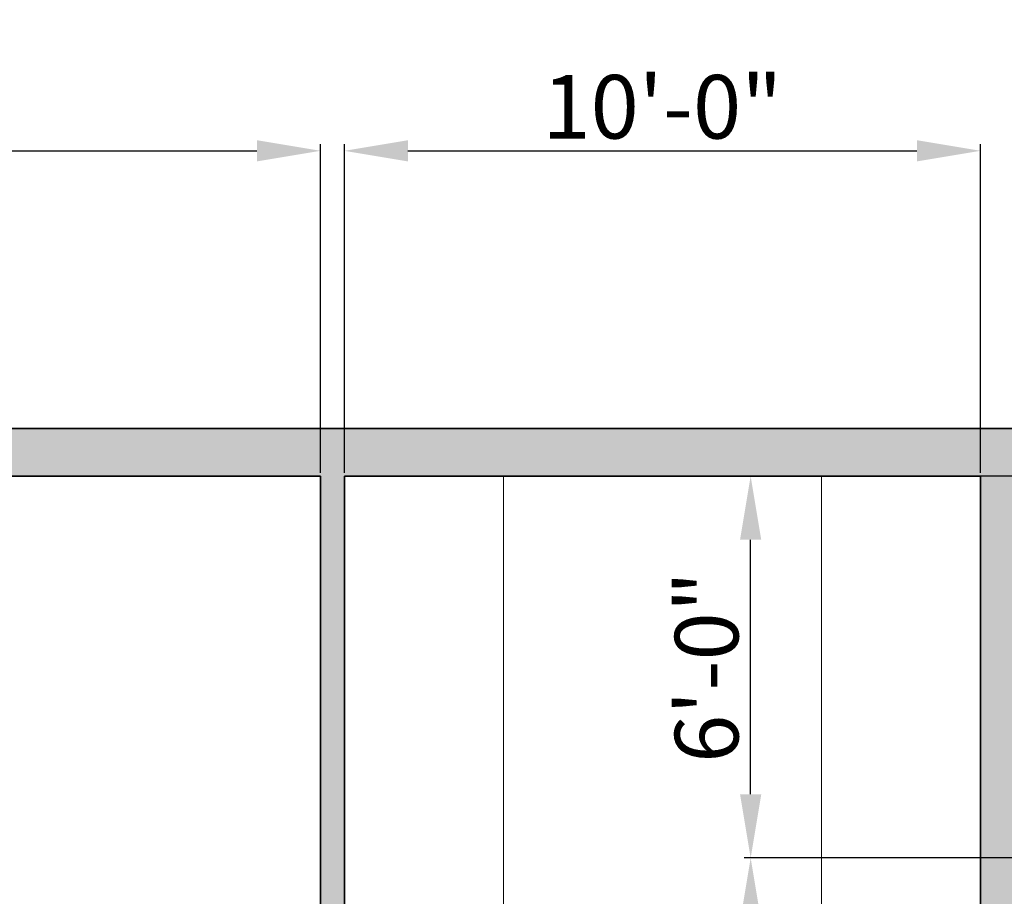
# Model space of a CAD drawing. Units: inches. Extents: x 2083 to 3317, y 1141 to 2115.
# Tile 105 of 256: x 2415 to 2600, y 1933 to 2098. Entities that reach past the tile are written whole.
import ezdxf

# ---------------------------------------------------------------- set-up
doc = ezdxf.new("R2010")
doc.units = ezdxf.units.IN
for name, color, linetype, lineweight in [('A-ANNO-DIMS', 2, 'Continuous', 18), ('A-FLOR-CASE', 8, 'Continuous', 18), ('A-WALL', 7, 'Continuous', 35)]:
    doc.layers.add(name, color=color, linetype=linetype, lineweight=lineweight)
doc.layers.add('A-WALL-PATT', color=251, linetype='Continuous', lineweight=13, true_color=0x636466)
doc.styles.get("Standard").update_dxf_attribs({"font": 'arial.ttf'})
doc.dimstyles.new('ISO-25', dxfattribs={"dimtxt": 12, "dimasz": 12, "dimexe": 1.25, "dimexo": 0.625, "dimtad": 1, "dimlunit": 3, "dimtxsty": 'Standard', "dimcen": 2.5, "dimadec": 0, "dimazin": 0, "dimtfac": 1, "dimtmove": 0, "dimatfit": 3, "dimfxl": 1, "dimarcsym": 0})

# ---------------------------------------------------------------- blocks, each defined once
blk = doc.blocks.new('*D36')
at = {"layer": 'A-ANNO-DIMS', "color": 0, "lineweight": -2, "transparency": 16777216}
for p, q in [((2235.96, 2012.39), (2235.96, 2074.36)), ((2247.96, 2073.11), (2459.46, 2073.11)), ((2471.46, 2012.39), (2471.46, 2074.36))]:
    blk.add_line(p, q, dxfattribs=at)
at = {"layer": 'A-ANNO-DIMS', "color": 0, "transparency": 16777216}
for points in [[(2247.96, 2075.11), (2247.96, 2071.11), (2235.96, 2073.11)], [(2459.46, 2075.11), (2459.46, 2071.11), (2471.46, 2073.11)]]:
    blk.add_solid(points, dxfattribs=at)
at = {"layer": 'Defpoints', "color": 0, "transparency": 16777216}
for p in [(2471.46, 2073.11), (2235.96, 2011.76), (2471.46, 2011.76)]:
    blk.add_point(p, dxfattribs=at)
at = {"layer": 'A-ANNO-DIMS', "color": 0, "transparency": 16777216, "insert": (2353.71, 2079.94), "char_height": 12, "attachment_point": 5}
blk.add_mtext('19\'-7 1/2"', dxfattribs=at)
blk = doc.blocks.new('*D37')
at = {"layer": 'A-ANNO-DIMS', "color": 0, "lineweight": -2, "transparency": 16777216}
for p, q in [((2475.96, 2012.39), (2475.96, 2074.36)), ((2487.96, 2073.11), (2583.96, 2073.11)), ((2595.96, 2012.39), (2595.96, 2074.36))]:
    blk.add_line(p, q, dxfattribs=at)
at = {"layer": 'A-ANNO-DIMS', "color": 0, "transparency": 16777216}
for points in [[(2487.96, 2075.11), (2487.96, 2071.11), (2475.96, 2073.11)], [(2583.96, 2075.11), (2583.96, 2071.11), (2595.96, 2073.11)]]:
    blk.add_solid(points, dxfattribs=at)
at = {"layer": 'Defpoints', "color": 0, "transparency": 16777216}
for p in [(2595.96, 2073.11), (2475.96, 2011.76), (2595.96, 2011.76)]:
    blk.add_point(p, dxfattribs=at)
at = {"layer": 'A-ANNO-DIMS', "color": 0, "transparency": 16777216, "insert": (2535.96, 2079.86), "char_height": 12, "attachment_point": 5}
blk.add_mtext('10\'-0"', dxfattribs=at)
blk = doc.blocks.new('*D50')
at = {"layer": 'A-ANNO-DIMS', "color": 0, "lineweight": -2, "transparency": 16777216}
for p, q in [((2604.33, 1939.76), (2551.36, 1939.76)), ((2552.61, 1807.76), (2552.61, 1927.76)), ((2604.33, 1795.76), (2551.36, 1795.76))]:
    blk.add_line(p, q, dxfattribs=at)
at = {"layer": 'A-ANNO-DIMS', "color": 0, "transparency": 16777216}
for points in [[(2550.61, 1927.76), (2554.61, 1927.76), (2552.61, 1939.76)], [(2550.61, 1807.76), (2554.61, 1807.76), (2552.61, 1795.76)]]:
    blk.add_solid(points, dxfattribs=at)
at = {"layer": 'Defpoints', "color": 0, "transparency": 16777216}
for p in [(2552.61, 1939.76), (2604.96, 1939.76), (2604.96, 1795.76)]:
    blk.add_point(p, dxfattribs=at)
at = {"layer": 'A-ANNO-DIMS', "color": 0, "transparency": 16777216, "insert": (2545.86, 1867.76), "char_height": 12, "attachment_point": 5, "rotation": 90}
blk.add_mtext('12\'-0"', dxfattribs=at)
blk = doc.blocks.new('*D51')
at = {"layer": 'A-ANNO-DIMS', "color": 0, "lineweight": -2, "transparency": 16777216}
for p, q in [((2604.33, 2011.76), (2551.36, 2011.76)), ((2552.61, 1951.76), (2552.61, 1999.76)), ((2604.33, 1939.76), (2551.36, 1939.76))]:
    blk.add_line(p, q, dxfattribs=at)
at = {"layer": 'A-ANNO-DIMS', "color": 0, "transparency": 16777216}
for points in [[(2550.61, 1999.76), (2554.61, 1999.76), (2552.61, 2011.76)], [(2550.61, 1951.76), (2554.61, 1951.76), (2552.61, 1939.76)]]:
    blk.add_solid(points, dxfattribs=at)
at = {"layer": 'Defpoints', "color": 0, "transparency": 16777216}
for p in [(2552.61, 2011.76), (2604.96, 2011.76), (2604.96, 1939.76)]:
    blk.add_point(p, dxfattribs=at)
at = {"layer": 'A-ANNO-DIMS', "color": 0, "transparency": 16777216, "insert": (2545.86, 1975.76), "char_height": 12, "attachment_point": 5, "rotation": 90}
blk.add_mtext('6\'-0"', dxfattribs=at)

msp = doc.modelspace()

# ---------------------------------------------------------------- hatches: boundary and pattern name
at = {"layer": 'A-WALL-PATT'}
h = msp.add_hatch(color=256, dxfattribs=at)
h.dxf.hatch_style = 1
h.paths.add_polyline_path([(3126.96, 2020.761), (2748.96, 2020.761), (2604.96, 2020.761), (2226.96, 2020.761), (2226.96, 1702.761), (2466.96, 1702.761), (2466.96, 1582.761), (2418.96, 1582.761), (2418.96, 1477.761), (2226.96, 1477.761), (2226.96, 1263.261), (2544.96, 1263.261), (2544.96, 1411.761), (2604.96, 1411.761), (2685.96, 1411.761), (2685.96, 1420.761), (2604.96, 1420.761), (2604.96, 1573.761), (2604.96, 1702.761), (2604.96, 2011.761), (2748.96, 2011.761), (2748.96, 1702.761), (2862.96, 1702.761), (2862.96, 1621.761), (2871.96, 1621.761), (2871.96, 1702.761), (2883.96, 1702.761), (2883.96, 1706.939, -0.0264593), (2883.96, 1711.761), (2757.96, 1711.761), (2757.96, 1807.761), (2787.96, 1807.761), (2787.96, 1812.261), (2757.96, 1812.261), (2757.96, 2011.761), (2877.96, 2011.761), (2877.96, 1812.261), (2847.96, 1812.261), (2847.96, 1807.761), (2889.836, 1807.761), (2889.836, 1812.261), (2882.46, 1812.261), (2882.46, 2011.761), (3117.96, 2011.761), (3117.96, 1812.261), (2937.836, 1812.261), (2937.836, 1807.761), (2995.71, 1807.761), (2995.71, 1796.118), (3000.21, 1796.118), (3000.21, 1807.761), (3117.96, 1807.761), (3117.96, 1711.761), (3000.21, 1711.761), (3000.21, 1760.118), (2998.573, 1760.118, -0.020711), (2995.71, 1760.118), (2995.71, 1711.761), (2931.96, 1711.761), (2931.96, 1702.761), (3126.96, 1702.761)])
h.paths.add_polyline_path([(2471.46, 2011.761), (2471.46, 1810.011), (2462.717, 1810.011), (2462.717, 1805.511), (2505.96, 1805.511), (2505.96, 1810.011), (2475.96, 1810.011), (2475.96, 2011.761), (2595.96, 2011.761), (2595.96, 1810.011), (2565.96, 1810.011), (2565.96, 1805.511), (2595.96, 1805.511), (2595.96, 1711.761), (2235.96, 1711.761), (2235.96, 1805.511), (2353.71, 1805.511), (2353.71, 1796.054), (2358.21, 1796.054), (2358.21, 1805.511), (2414.717, 1805.511), (2414.717, 1810.011), (2235.96, 1810.011), (2235.96, 2011.761)], flags=16)
h.paths.add_polyline_path([(2270.205, 1994.61), (2270.205, 1970.61), (2246.205, 1970.61), (2246.205, 1994.61)], flags=0)
edge = h.paths.add_edge_path(flags=0)
edge.add_ellipse((2332.027, 1899.798), major_axis=(-3.043, 3.043), ratio=0.1682525, start_angle=-161.33217, end_angle=-156.30711, ccw=False)
edge.add_ellipse((2333.082, 1898.744), major_axis=(-1.055, 1.055), ratio=0.4535321, start_angle=-123.37102, end_angle=-94.15911)
edge = h.paths.add_edge_path(flags=0)
edge.add_ellipse((2332.027, 1968.876), major_axis=(3.043, 3.043), ratio=0.1682525, start_angle=18.66783, end_angle=23.69289)
edge.add_spline(control_points=[(2332.926, 1970.691), (2332.227, 1970.336), (2330.894, 1969.659), (2328.413, 1970.932), (2327.204, 1967.749), (2324.71, 1969.956), (2322.533, 1967.012), (2320.013, 1971.296), (2317.68, 1968.158), (2316.041, 1967.102), (2315.427, 1966.81)], knot_values=[0, 0, 0, 0, 2.2670587, 4.3245589, 6.6855835, 8.8786411, 11.121502, 14.300359, 17.7552837, 19.732645, 19.732645, 19.732645, 19.732645], degree=3, periodic=0)
edge.add_ellipse((2332.027, 1968.876), major_axis=(3.043, 3.043), ratio=0.1682525, start_angle=18.66783, end_angle=23.69289, ccw=False)
edge.add_ellipse((2333.082, 1969.931), major_axis=(1.055, 1.055), ratio=0.4535321, start_angle=56.62898, end_angle=85.84089, ccw=False)
edge = h.paths.add_edge_path(flags=0)
edge.add_spline(control_points=[(2296.428, 1967.988), (2293.628, 1965.336), (2287.704, 1959.727), (2299.744, 1949.996), (2294.533, 1935.669), (2290.573, 1920.604), (2293.394, 1909.974), (2296.185, 1904.967)], knot_values=[0.0991853, 0.0991853, 0.0991853, 0.0991853, 0.3453009, 0.6198217, 0.9826526, 1.3860932, 1.8105546, 1.8105546, 1.8105546, 1.8105546], degree=3, periodic=0)
edge.add_spline(control_points=[(2296.185, 1904.967), (2297.384, 1902.619), (2298.001, 1901.949), (2298.553, 1901.468)], knot_values=[0.0062457, 0.0062457, 0.0062457, 0.0062457, 0.0554759, 0.0554759, 0.0554759, 0.0554759], degree=3, periodic=0)
edge.add_spline(control_points=[(2298.553, 1901.468), (2297.259, 1900.923), (2295.225, 1900.232), (2293.06, 1900.614), (2292.101, 1900.788), (2292.09, 1900.791)], knot_values=[0.3128349, 0.3128349, 0.3128349, 0.3128349, 0.4017797, 0.4749867, 0.4759027, 0.4759027, 0.4759027, 0.4759027], degree=3, periodic=0)
edge.add_arc((2292.794, 1904.664), 3.937, 215.4209, 259.69818, ccw=False)
edge.add_spline(control_points=[(2289.585, 1902.382), (2289.477, 1902.535), (2289.368, 1902.688), (2289.261, 1902.841)], knot_values=[0.1028719, 0.1028719, 0.1028719, 0.1028719, 0.1168958, 0.1168958, 0.1168958, 0.1168958], degree=3, periodic=0)
edge.add_spline(control_points=[(2289.261, 1902.841), (2288.687, 1902.55), (2287.64, 1902.02), (2285.881, 1901.874), (2283.853, 1901.504), (2281.72, 1899.711), (2278.467, 1899.493), (2276.157, 1901.883), (2272.259, 1899.804), (2267.778, 1901.843), (2262.244, 1900.184), (2257.415, 1901.782), (2254.318, 1900.726), (2253.178, 1900.337)], knot_values=[0, 0, 0, 0, 1.9079767, 3.4771759, 5.261074, 7.9728515, 11.6802485, 13.7179214, 16.9395917, 22.789562, 27.5025027, 33.5952153, 37.1456181, 37.1456181, 37.1456181, 37.1456181], degree=3, periodic=0)
edge.add_line((2253.178, 1900.337), (2250.244, 1902.841))
edge.add_line((2250.244, 1902.841), (2250.244, 1965.833))
edge.add_line((2250.244, 1965.833), (2253.178, 1968.337))
edge.add_spline(control_points=[(2253.178, 1968.337), (2254.318, 1967.948), (2257.415, 1966.892), (2262.244, 1968.49), (2267.778, 1966.831), (2271.527, 1968.537), (2273.876, 1967.828), (2274.207, 1967.728)], knot_values=[0, 0, 0, 0, 0.0901802, 0.2449351, 0.3646438, 0.5132331, 0.5378548, 0.5378548, 0.5378548, 0.5378548], degree=3, periodic=0)
edge.add_arc((2274.353, 1963.793), 3.937, 72.05113, 92.12795, ccw=False)
edge.add_arc((2281.297, 1985.23), 18.596, 252.05113, 288.56572)
edge.add_arc((2292.317, 1956.029), 12.646, 71.02679, 113.77822, ccw=False)
edge = h.paths.add_edge_path(flags=0)
edge.add_spline(control_points=[(2274.899, 1951.856), (2275.066, 1951.617), (2275.233, 1951.377), (2275.398, 1951.136)], knot_values=[1.4099157, 1.4099157, 1.4099157, 1.4099157, 1.4315903, 1.4315903, 1.4315903, 1.4315903], degree=3, periodic=0)
edge.add_spline(control_points=[(2275.398, 1951.136), (2275.792, 1950.562), (2276.179, 1949.984), (2276.546, 1949.397)], knot_values=[1.3582378, 1.3582378, 1.3582378, 1.3582378, 1.4099157, 1.4099157, 1.4099157, 1.4099157], degree=3, periodic=0)
edge.add_line((2276.546, 1949.397), (2277.437, 1947.862))
edge.add_spline(control_points=[(2277.437, 1947.862), (2276.304, 1945.673), (2274.64, 1942.427), (2274.632, 1938.094), (2272.799, 1930.852), (2274.356, 1943.897), (2275.948, 1947.923), (2276.546, 1949.397)], knot_values=[0.0056315, 0.0056315, 0.0056315, 0.0056315, 0.1860139, 0.2660015, 0.3570872, 0.5963902, 0.7397317, 0.7397317, 0.7397317, 0.7397317], degree=3, periodic=0)
edge.add_spline(control_points=[(2276.546, 1949.397), (2276.179, 1949.984), (2275.792, 1950.562), (2275.398, 1951.136)], knot_values=[1.3582378, 1.3582378, 1.3582378, 1.3582378, 1.4099157, 1.4099157, 1.4099157, 1.4099157], degree=3, periodic=0)
edge.add_spline(control_points=[(2275.398, 1951.136), (2274.943, 1950.08), (2274.208, 1948.025), (2273.935, 1944.851), (2272.469, 1937.627), (2273.466, 1945.696), (2274.701, 1951.059), (2274.899, 1951.856)], knot_values=[0.1043639, 0.1043639, 0.1043639, 0.1043639, 0.1896363, 0.2696239, 0.3607096, 0.6000126, 0.6446217, 0.6446217, 0.6446217, 0.6446217], degree=3, periodic=0)
h.paths.add_polyline_path([(2269.168, 1963.128, -0.3575267), (2268.171, 1960.976, -0.0925607), (2268.171, 1939.436, -0.3575267), (2269.168, 1937.285, -0.3575267), (2267.016, 1938.282, -0.1647847), (2254.686, 1938.282, -0.3575267), (2252.534, 1937.285, -0.3575267), (2253.531, 1939.436, -0.0925607), (2253.531, 1960.976, -0.3575267), (2252.534, 1963.128, -0.3575267), (2254.686, 1962.131, -0.1647847), (2267.016, 1962.131, -0.3575267)], flags=0)
h.paths.add_polyline_path([(2248.874, 1967.802), (2248.874, 1957.028), (2249.458, 1957.028), (2249.458, 1911.647), (2248.874, 1911.647), (2248.874, 1900.873), (2246.512, 1900.873, 0.1973271), (2244.15, 1902.457), (2244.15, 1966.218, 0.1973271), (2246.512, 1967.802)], flags=0)
h.paths.add_polyline_path([(2269.168, 1931.389, -0.3575267), (2268.171, 1929.238, -0.0925607), (2268.171, 1907.698, -0.3575267), (2269.168, 1905.547, -0.3575267), (2267.016, 1906.544, -0.1647847), (2254.686, 1906.544, -0.3575267), (2252.534, 1905.547, -0.3575267), (2253.531, 1907.698, -0.0925607), (2253.531, 1929.238, -0.3575267), (2252.534, 1931.389, -0.3575267), (2254.686, 1930.392, -0.1647847), (2267.016, 1930.392, -0.3575267)], flags=0)
edge = h.paths.add_edge_path(flags=0)
edge.add_spline(control_points=[(2276.197, 1906.724), (2276.168, 1909.029), (2276.114, 1913.372), (2270.598, 1924.925), (2273.905, 1919.013), (2275.922, 1916.262), (2275.475, 1912.402), (2277.258, 1910.381), (2276.696, 1908.225), (2276.646, 1906.813), (2276.618, 1906.008)], knot_values=[0, 0, 0, 0, 8.6102597, 16.2212739, 18.8430575, 23.8048978, 27.4408283, 29.3561016, 31.2034776, 33.6506866, 33.6506866, 33.6506866, 33.6506866], degree=3, periodic=0)
edge.add_spline(control_points=[(2276.618, 1906.008), (2276.623, 1905.624), (2276.498, 1904.629), (2275.442, 1903.855), (2274.937, 1903.08), (2274.859, 1902.841)], knot_values=[0.1564884, 0.1564884, 0.1564884, 0.1564884, 0.1843975, 0.2313765, 0.2505985, 0.2505985, 0.2505985, 0.2505985], degree=3, periodic=0)
edge.add_line((2274.859, 1902.841), (2276.506, 1902.841))
edge.add_spline(control_points=[(2276.506, 1902.841), (2276.788, 1903.085), (2277.665, 1904.125), (2278.25, 1904.341), (2277.654, 1908.527), (2278.156, 1906.228), (2278.1, 1905.286), (2278.847, 1904.069), (2277.857, 1903.415), (2277.874, 1902.991), (2277.904, 1902.841)], knot_values=[0.0595743, 0.0595743, 0.0595743, 0.0595743, 0.0807529, 0.1037415, 0.1697201, 0.1760361, 0.2071372, 0.2404744, 0.2623409, 0.2736605, 0.2736605, 0.2736605, 0.2736605], degree=3, periodic=0)
edge.add_line((2277.904, 1902.841), (2280.03, 1902.841))
edge.add_spline(control_points=[(2280.03, 1902.841), (2279.888, 1903.088), (2279.499, 1903.982), (2280.152, 1905.939), (2278.104, 1909.658), (2279.762, 1907.185), (2280.328, 1904.875), (2280.485, 1903.49), (2281.463, 1903.249), (2281.758, 1902.936), (2281.834, 1902.841)], knot_values=[0.013856, 0.013856, 0.013856, 0.013856, 0.0348738, 0.0888667, 0.1078792, 0.1267378, 0.158714, 0.1937575, 0.2174868, 0.2267221, 0.2267221, 0.2267221, 0.2267221], degree=3, periodic=0)
edge.add_spline(control_points=[(2281.834, 1902.841), (2281.788, 1902.827), (2281.647, 1902.783), (2281.396, 1902.859), (2281.088, 1902.985), (2280.721, 1903.061), (2280.333, 1903.026), (2280.125, 1902.899), (2280.03, 1902.841)], knot_values=[0, 0, 0, 0, 0.1441304, 0.435517, 0.7492759, 1.1530457, 1.5483707, 1.878348, 1.878348, 1.878348, 1.878348], degree=3, periodic=0)
edge.add_line((2280.03, 1902.841), (2277.904, 1902.841))
edge.add_spline(control_points=[(2277.904, 1902.841), (2277.893, 1902.796), (2277.865, 1902.68), (2277.607, 1902.687), (2277.274, 1902.801), (2276.838, 1902.62), (2276.584, 1902.789), (2276.506, 1902.841)], knot_values=[0, 0, 0, 0, 0.1271885, 0.3261988, 0.6280094, 1.2435704, 1.5153306, 1.5153306, 1.5153306, 1.5153306], degree=3, periodic=0)
edge.add_line((2276.506, 1902.841), (2274.859, 1902.841))
edge.add_spline(control_points=[(2274.859, 1902.841), (2274.814, 1902.899), (2274.725, 1903.013), (2274.493, 1903.119), (2274.244, 1902.961), (2273.937, 1903.185), (2273.614, 1902.983), (2273.408, 1902.883), (2273.322, 1902.841)], knot_values=[0, 0, 0, 0, 0.2184302, 0.4369566, 0.6879766, 0.9903786, 1.3983955, 1.6918498, 1.6918498, 1.6918498, 1.6918498], degree=3, periodic=0)
edge.add_spline(control_points=[(2273.322, 1902.841), (2273.617, 1903.446), (2274.274, 1904.538), (2276.027, 1904.574), (2276.207, 1906.584), (2276.197, 1906.724)], knot_values=[0.0122268, 0.0122268, 0.0122268, 0.0122268, 0.0594721, 0.1062177, 0.134458, 0.134458, 0.134458, 0.134458], degree=3, periodic=0)
h.paths.add_polyline_path([(2270.776, 1897.79), (2270.776, 1873.79), (2246.776, 1873.79), (2246.776, 1897.79)], flags=0)
h.paths.add_polyline_path([(2353.71, 1760.005), (2353.71, 1760.054), (2358.21, 1760.054, -0.033729)], flags=0)
h.paths.add_polyline_path([(2321.819, 1737.529), (2341.995, 1737.529, -0.4142136), (2343.203, 1736.321), (2343.203, 1721.021, -0.4142136), (2341.995, 1719.813), (2321.819, 1719.813, -0.4142136), (2320.611, 1721.021), (2320.611, 1736.321, -0.4142136)], flags=0)
h.paths.add_polyline_path([(2324.235, 1736.321), (2339.579, 1736.321, -0.4142136), (2341.995, 1733.905), (2341.995, 1725.45, -0.4142136), (2339.579, 1723.034), (2333.681, 1723.034), (2333.845, 1722.045, -0.8706461), (2335.425, 1721.826, -0.767327), (2333.923, 1721.423), (2331.291, 1721.423, -0.767327), (2329.788, 1721.826, -0.8706461), (2331.368, 1722.045), (2331.533, 1723.034), (2324.235, 1723.034, -0.4142136), (2321.819, 1725.45), (2321.819, 1733.905, -0.4142136)], flags=0)
h.paths.add_polyline_path([(2570.484, 1928.615), (2589.684, 1928.615), (2590.169, 1928.615), (2590.169, 1904.993), (2570.484, 1904.993)], flags=0)
h.paths.add_polyline_path([(2574.447, 1927.264, -1), (2572.829, 1927.264, -1)], flags=0)
h.paths.add_polyline_path([(2573.09, 1926.941), (2573.925, 1927.776), (2574.148, 1927.553), (2573.313, 1926.718)], flags=0)
h.paths.add_polyline_path([(2578.779, 1919.73, -1), (2571.592, 1919.73, -1)], flags=0)
h.paths.add_polyline_path([(2578.385, 1919.73, -1), (2571.985, 1919.73, -1)], flags=0)
h.paths.add_polyline_path([(2331.596, 1729.476, -1), (2333.618, 1729.476, -1)], flags=0)
h.paths.add_polyline_path([(2578.034, 1927.264, -1), (2576.416, 1927.264, -1)], flags=0)
h.paths.add_polyline_path([(2576.689, 1927.531), (2576.912, 1927.754), (2577.747, 1926.919), (2577.524, 1926.696)], flags=0)
h.paths.add_polyline_path([(2578.139, 1909.86, -1), (2572.232, 1909.86, -1)], flags=0)
h.paths.add_polyline_path([(2577.745, 1909.86, -1), (2572.625, 1909.86, -1)], flags=0)
h.paths.add_polyline_path([(2583.798, 1927.264, -1), (2582.179, 1927.264, -1)], flags=0)
h.paths.add_polyline_path([(2582.719, 1927.754), (2583.554, 1926.919), (2583.331, 1926.696), (2582.496, 1927.531)], flags=0)
h.paths.add_polyline_path([(2582.496, 1927.531), (2582.719, 1927.754), (2583.554, 1926.919), (2583.331, 1926.696)], flags=0)
h.paths.add_polyline_path([(2587.739, 1920.53, -1), (2581.832, 1920.53, -1)], flags=0)
h.paths.add_polyline_path([(2587.345, 1920.53, -1), (2582.225, 1920.53, -1)], flags=0)
h.paths.add_polyline_path([(2587.385, 1927.264, -1), (2585.766, 1927.264, -1)], flags=0)
h.paths.add_polyline_path([(2586.082, 1926.98), (2586.917, 1927.815), (2587.14, 1927.593), (2586.305, 1926.758)], flags=0)
h.paths.add_polyline_path([(2588.379, 1910.66, -1), (2581.192, 1910.66, -1)], flags=0)
h.paths.add_polyline_path([(2587.985, 1910.66, -1), (2581.585, 1910.66, -1)], flags=0)
h.paths.add_polyline_path([(2417.168, 1729.478), (2437.344, 1729.478, -0.4142136), (2438.552, 1728.27), (2438.552, 1712.969, -0.4142136), (2437.344, 1711.761), (2417.168, 1711.761, -0.4142136), (2415.96, 1712.969), (2415.96, 1728.27, -0.4142136)], flags=0)
h.paths.add_polyline_path([(2419.584, 1728.27), (2434.928, 1728.27, -0.4142136), (2437.344, 1725.854), (2437.344, 1717.398, -0.4142136), (2434.928, 1714.983), (2429.029, 1714.983), (2429.194, 1713.994, -0.8706461), (2430.774, 1713.775, -0.767327), (2429.271, 1713.372), (2426.64, 1713.372, -0.767327), (2425.137, 1713.775, -0.8706461), (2426.717, 1713.994), (2426.882, 1714.983), (2419.584, 1714.983, -0.4142136), (2417.168, 1717.398), (2417.168, 1725.854, -0.4142136)], flags=0)
h.paths.add_polyline_path([(2419.584, 1728.27), (2434.928, 1728.27, -0.4142136), (2437.344, 1725.854), (2437.344, 1717.398, -0.4142136), (2434.928, 1714.983), (2429.029, 1714.983), (2428.358, 1719.009), (2427.553, 1719.009), (2426.882, 1714.983), (2419.584, 1714.983, -0.4142136), (2417.168, 1717.398), (2417.168, 1725.854, -0.4142136)], flags=0)
h.paths.add_polyline_path([(2426.944, 1721.425, -1), (2428.967, 1721.425, -1)], flags=0)
h.paths.add_polyline_path([(2475.96, 1702.761), (2595.96, 1702.761), (2595.96, 1582.761), (2475.96, 1582.761)], flags=16)
h.paths.add_polyline_path([(2427.96, 1573.761), (2595.96, 1573.761), (2595.96, 1468.761), (2595.96, 1420.761), (2384.46, 1420.761), (2384.46, 1468.761), (2427.96, 1468.761)], flags=16)
h.paths.add_polyline_path([(2379.96, 1468.761), (2379.96, 1420.761), (2235.96, 1420.761), (2235.96, 1468.761)], flags=16)
h.paths.add_polyline_path([(2317.816, 1466.696), (2337.992, 1466.696, -0.4142136), (2339.2, 1465.488), (2339.2, 1450.187, -0.4142136), (2337.992, 1448.979), (2317.816, 1448.979, -0.4142136), (2316.608, 1450.187), (2316.608, 1465.488, -0.4142136)], flags=0)
h.paths.add_polyline_path([(2320.232, 1465.488), (2335.576, 1465.488, -0.4142136), (2337.992, 1463.072), (2337.992, 1454.616, -0.4142136), (2335.576, 1452.2), (2329.677, 1452.2), (2329.842, 1451.212, -0.8706461), (2331.422, 1450.992, -0.767327), (2329.92, 1450.59), (2327.288, 1450.59, -0.767327), (2325.785, 1450.992, -0.8706461), (2327.365, 1451.212), (2327.53, 1452.2), (2320.232, 1452.2, -0.4142136), (2317.816, 1454.616), (2317.816, 1463.072, -0.4142136)], flags=0)
h.paths.add_polyline_path([(2320.232, 1465.488), (2335.576, 1465.488, -0.4142136), (2337.992, 1463.072), (2337.992, 1454.616, -0.4142136), (2335.576, 1452.2), (2329.677, 1452.2), (2329.006, 1456.227), (2328.201, 1456.227), (2327.53, 1452.2), (2320.232, 1452.2, -0.4142136), (2317.816, 1454.616), (2317.816, 1463.072, -0.4142136)], flags=0)
h.paths.add_polyline_path([(2327.593, 1458.643, -1), (2329.615, 1458.643, -1)], flags=0)
h.paths.add_polyline_path([(2244.412, 1433.34), (2241.921, 1433.34, -0.4142136), (2240.018, 1435.244), (2240.018, 1440.953, -0.4142105), (2241.921, 1442.856), (2244.412, 1442.856, -1.9764724)], flags=0)
h.paths.add_polyline_path([(2245.357, 1434.398, -0.4142136), (2245.357, 1441.799, -2.1440985)], flags=0)
h.paths.add_polyline_path([(2535.96, 1416.261), (2535.96, 1272.261), (2235.96, 1272.261), (2235.96, 1416.261)], flags=16)
h.paths.add_polyline_path([(2260.12, 1384.293), (2260.12, 1362.039), (2237.865, 1362.039), (2237.865, 1384.293)], flags=0)
edge = h.paths.add_edge_path(flags=0)
edge.add_line((2318.252, 1362.093), (2318.146, 1362.001))
edge.add_ellipse((2317.445, 1360.431), major_axis=(2.822, 2.822), ratio=0.1682525, start_angle=18.66783, end_angle=20.94813, ccw=False)
edge.add_ellipse((2318.423, 1361.409), major_axis=(0.978, 0.978), ratio=0.4535321, start_angle=56.62898, end_angle=70.2262, ccw=False)
edge = h.paths.add_edge_path(flags=0)
edge.add_line((2319.107, 1295.571), (2319.015, 1295.677))
edge.add_ellipse((2317.445, 1296.378), major_axis=(-2.822, 2.822), ratio=0.1682525, start_angle=-161.33217, end_angle=-159.05187, ccw=False)
edge.add_ellipse((2318.423, 1295.4), major_axis=(-0.978, 0.978), ratio=0.4535321, start_angle=-123.37102, end_angle=-109.7738)
edge = h.paths.add_edge_path(flags=0)
edge.add_spline(control_points=[(2284.21, 1301.17), (2284.581, 1300.445), (2284.891, 1299.892), (2285.16, 1299.461)], knot_values=[0.0390658, 0.0390658, 0.0390658, 0.0390658, 0.0554759, 0.0554759, 0.0554759, 0.0554759], degree=3, periodic=0)
edge.add_line((2285.16, 1299.461), (2284.21, 1301.17))
edge = h.paths.add_edge_path(flags=0)
edge.add_line((2280.412, 1297.298), (2283.37, 1297.036))
edge.add_line((2283.37, 1297.036), (2286.406, 1297.926))
edge.add_spline(control_points=[(2286.406, 1297.926), (2285.305, 1297.463), (2284.345, 1297.129), (2283.37, 1297.036)], knot_values=[0.3943688, 0.3943688, 0.3943688, 0.3943688, 0.4759027, 0.4759027, 0.4759027, 0.4759027], degree=3, periodic=0)
edge.add_spline(control_points=[(2283.37, 1297.036), (2283.281, 1297.028), (2282.316, 1296.957), (2281.313, 1297.134), (2280.423, 1297.296), (2280.412, 1297.298)], knot_values=[0.3128349, 0.3128349, 0.3128349, 0.3128349, 0.3202458, 0.3934528, 0.3943688, 0.3943688, 0.3943688, 0.3943688], degree=3, periodic=0)
edge = h.paths.add_edge_path(flags=0)
edge.add_line((2284.436, 1359.607), (2280.446, 1355.328))
edge.add_line((2280.446, 1355.328), (2279.58, 1351.018))
edge.add_line((2279.58, 1351.018), (2282.413, 1346.58))
edge.add_spline(control_points=[(2282.413, 1346.58), (2283.153, 1345.589), (2284.253, 1344.029), (2284.801, 1342.387), (2284.935, 1341.806)], knot_values=[1.2400982, 1.2400982, 1.2400982, 1.2400982, 1.3328922, 1.3827123, 1.3827123, 1.3827123, 1.3827123], degree=3, periodic=0)
edge.add_spline(control_points=[(2284.935, 1341.806), (2285.319, 1340.141), (2285.233, 1338.409), (2284.91, 1336.654)], knot_values=[1.0974841, 1.0974841, 1.0974841, 1.0974841, 1.2400982, 1.2400982, 1.2400982, 1.2400982], degree=3, periodic=0)
edge.add_spline(control_points=[(2284.91, 1336.654), (2284.587, 1334.899), (2284.027, 1333.12), (2283.463, 1331.361)], knot_values=[0.9548699, 0.9548699, 0.9548699, 0.9548699, 1.0974841, 1.0974841, 1.0974841, 1.0974841], degree=3, periodic=0)
edge.add_line((2283.463, 1331.361), (2281.89, 1326.153))
edge.add_line((2281.89, 1326.153), (2280.756, 1321.056))
edge.add_line((2280.756, 1321.056), (2280.299, 1316.002))
edge.add_line((2280.299, 1316.002), (2280.716, 1310.95))
edge.add_line((2280.716, 1310.95), (2282.028, 1305.972))
edge.add_line((2282.028, 1305.972), (2284.21, 1301.17))
edge.add_spline(control_points=[(2284.21, 1301.17), (2283.341, 1302.73), (2282.612, 1304.336), (2282.028, 1305.972)], knot_values=[0.0991853, 0.0991853, 0.0991853, 0.0991853, 0.2417994, 0.2417994, 0.2417994, 0.2417994], degree=3, periodic=0)
edge.add_spline(control_points=[(2282.028, 1305.972), (2281.444, 1307.608), (2281.005, 1309.273), (2280.716, 1310.95)], knot_values=[0.2417994, 0.2417994, 0.2417994, 0.2417994, 0.3844135, 0.3844135, 0.3844135, 0.3844135], degree=3, periodic=0)
edge.add_spline(control_points=[(2280.716, 1310.95), (2280.433, 1312.588), (2280.289, 1314.277), (2280.299, 1315.962), (2280.299, 1316.002)], knot_values=[0.3844135, 0.3844135, 0.3844135, 0.3844135, 0.5236467, 0.5270276, 0.5270276, 0.5270276, 0.5270276], degree=3, periodic=0)
edge.add_spline(control_points=[(2280.299, 1316.002), (2280.312, 1317.687), (2280.478, 1319.368), (2280.756, 1321.056)], knot_values=[0.5270276, 0.5270276, 0.5270276, 0.5270276, 0.6696417, 0.6696417, 0.6696417, 0.6696417], degree=3, periodic=0)
edge.add_spline(control_points=[(2280.756, 1321.056), (2281.035, 1322.744), (2281.426, 1324.44), (2281.89, 1326.153)], knot_values=[0.6696417, 0.6696417, 0.6696417, 0.6696417, 0.8122558, 0.8122558, 0.8122558, 0.8122558], degree=3, periodic=0)
edge.add_spline(control_points=[(2281.89, 1326.153), (2282.264, 1327.533), (2282.788, 1329.262), (2283.353, 1331.018), (2283.463, 1331.361)], knot_values=[0.8122558, 0.8122558, 0.8122558, 0.8122558, 0.9270873, 0.9548699, 0.9548699, 0.9548699, 0.9548699], degree=3, periodic=0)
edge.add_line((2283.463, 1331.361), (2284.91, 1336.654))
edge.add_line((2284.91, 1336.654), (2284.935, 1341.806))
edge.add_line((2284.935, 1341.806), (2282.413, 1346.58))
edge.add_spline(control_points=[(2282.413, 1346.58), (2281.275, 1348.104), (2280.078, 1349.57), (2279.58, 1351.018)], knot_values=[1.3827123, 1.3827123, 1.3827123, 1.3827123, 1.5253264, 1.5253264, 1.5253264, 1.5253264], degree=3, periodic=0)
edge.add_spline(control_points=[(2279.58, 1351.018), (2279.443, 1351.415), (2279.136, 1352.857), (2279.735, 1354.29), (2280.446, 1355.328)], knot_values=[1.5253264, 1.5253264, 1.5253264, 1.5253264, 1.564439, 1.6679405, 1.6679405, 1.6679405, 1.6679405], degree=3, periodic=0)
edge.add_spline(control_points=[(2280.446, 1355.328), (2281.426, 1356.758), (2282.931, 1358.183), (2284.436, 1359.607)], knot_values=[1.6679405, 1.6679405, 1.6679405, 1.6679405, 1.8105546, 1.8105546, 1.8105546, 1.8105546], degree=3, periodic=0)
edge.add_arc((2280.623, 1348.518), 11.726, 71.02679, 113.77822)
edge.add_arc((2270.405, 1375.595), 17.244, 252.05113, 288.56572, ccw=False)
edge.add_arc((2263.966, 1355.718), 3.651, 72.05113, 92.12795)
edge.add_arc((2263.966, 1355.718), 3.651, 92.12795, 177.98513)
edge.add_spline(control_points=[(2260.318, 1355.846), (2260.26, 1354.221), (2260.551, 1350.187), (2262.999, 1346.766), (2264.473, 1344.649)], knot_values=[1.4315903, 1.4315903, 1.4315903, 1.4315903, 1.5641438, 1.7706953, 1.7706953, 1.7706953, 1.7706953], degree=3, periodic=0)
edge.add_line((2264.473, 1344.649), (2264.936, 1343.983))
edge.add_spline(control_points=[(2263.801, 1340.248), (2263.843, 1340.514), (2264.067, 1341.756), (2264.513, 1343.002), (2264.935, 1343.981)], knot_values=[0.5365702, 0.5365702, 0.5365702, 0.5365702, 0.5593494, 0.6446217, 0.6446217, 0.6446217, 0.6446217], degree=3, periodic=0)
edge.add_spline(control_points=[(2264.935, 1343.981), (2265.118, 1343.715), (2265.299, 1343.448), (2265.477, 1343.179)], knot_values=[1.3840767, 1.3840767, 1.3840767, 1.3840767, 1.4099157, 1.4099157, 1.4099157, 1.4099157], degree=3, periodic=0)
edge.add_spline(control_points=[(2265.477, 1343.179), (2265.655, 1342.911), (2265.829, 1342.641), (2265.999, 1342.369)], knot_values=[1.3582378, 1.3582378, 1.3582378, 1.3582378, 1.3840767, 1.3840767, 1.3840767, 1.3840767], degree=3, periodic=0)
edge.add_line((2265.999, 1342.369), (2266.826, 1340.946))
edge.add_spline(control_points=[(2266.826, 1340.946), (2268.894, 1337.09), (2271.398, 1325.843), (2270.516, 1310.569), (2275.919, 1301.861), (2277.79, 1299.199)], knot_values=[0.1168958, 0.1168958, 0.1168958, 0.1168958, 0.4729873, 1.0509689, 1.3137934, 1.3137934, 1.3137934, 1.3137934], degree=3, periodic=0)
edge.add_spline(control_points=[(2277.79, 1299.199), (2277.839, 1299.128), (2277.889, 1299.057), (2277.94, 1298.987)], knot_values=[0.1098839, 0.1098839, 0.1098839, 0.1098839, 0.1168958, 0.1168958, 0.1168958, 0.1168958], degree=3, periodic=0)
edge.add_line((2277.94, 1298.987), (2277.789, 1299.199))
edge.add_spline(control_points=[(2277.789, 1299.199), (2277.257, 1298.929), (2276.286, 1298.438), (2275.039, 1298.334), (2274.383, 1298.239), (2274.215, 1298.209)], knot_values=[33.1218702, 33.1218702, 33.1218702, 33.1218702, 35.0290557, 36.5982549, 37.1448269, 37.1448269, 37.1448269, 37.1448269], degree=3, periodic=0)
edge.add_line((2274.215, 1298.209), (2273.073, 1297.893))
edge.add_spline(control_points=[(2273.073, 1297.893), (2272.323, 1297.58), (2271.039, 1296.511), (2269.248, 1296.226), (2268.423, 1296.375)], knot_values=[26.5325843, 26.5325843, 26.5325843, 26.5325843, 29.198919, 31.8391012, 31.8391012, 31.8391012, 31.8391012], degree=3, periodic=0)
edge.add_line((2268.423, 1296.375), (2263.879, 1297.458))
edge.add_spline(control_points=[(2263.879, 1297.458), (2263.556, 1297.359), (2261.86, 1296.839), (2260.239, 1297.282), (2258.933, 1297.516)], knot_values=[15.9195506, 15.9195506, 15.9195506, 15.9195506, 16.9395917, 21.2260675, 21.2260675, 21.2260675, 21.2260675], degree=3, periodic=0)
edge.add_line((2258.933, 1297.516), (2254.055, 1297.329))
edge.add_spline(control_points=[(2254.055, 1297.329), (2253.756, 1297.296), (2252.114, 1297.165), (2250.462, 1297.544), (2249.13, 1297.668)], knot_values=[5.3065169, 5.3065169, 5.3065169, 5.3065169, 6.2764352, 10.6130337, 10.6130337, 10.6130337, 10.6130337], degree=3, periodic=0)
edge.add_line((2249.13, 1297.668), (2244.332, 1296.878))
edge.add_line((2244.332, 1296.878), (2241.611, 1299.199))
edge.add_line((2241.611, 1299.199), (2241.611, 1357.609))
edge.add_line((2241.611, 1357.609), (2244.332, 1359.931))
edge.add_line((2244.332, 1359.931), (2252.729, 1359.543))
edge.add_spline(control_points=[(2252.729, 1359.543), (2252.871, 1359.546), (2253.306, 1359.548), (2253.74, 1359.514), (2254.032, 1359.482)], knot_values=[0.233291, 0.233291, 0.233291, 0.233291, 0.2449351, 0.2689274, 0.2689274, 0.2689274, 0.2689274], degree=3, periodic=0)
edge.add_line((2254.032, 1359.482), (2259.587, 1359.416))
edge.add_spline(control_points=[(2259.587, 1359.416), (2260.677, 1359.629), (2262.073, 1359.897), (2263.524, 1359.459), (2263.83, 1359.366)], knot_values=[0.4225164, 0.4225164, 0.4225164, 0.4225164, 0.5132331, 0.5378548, 0.5378548, 0.5378548, 0.5378548], degree=3, periodic=0)
edge.add_arc((2263.966, 1355.718), 3.651, 72.05113, 92.12795, ccw=False)
edge.add_arc((2270.405, 1375.595), 17.244, 252.05113, 288.56572)
edge.add_arc((2280.623, 1348.518), 11.726, 71.02679, 113.77822, ccw=False)
h.paths.add_polyline_path([(2240.341, 1359.435), (2240.341, 1349.444), (2240.882, 1349.444), (2240.882, 1307.365), (2240.341, 1307.365), (2240.341, 1297.374), (2238.15, 1297.374, 0.1973271), (2235.96, 1298.843), (2235.96, 1357.966, 0.1973271), (2238.15, 1359.435)], flags=0)
h.paths.add_polyline_path([(2259.158, 1355.101, -0.3575267), (2258.233, 1353.106, -0.0925607), (2258.233, 1333.133, -0.3575267), (2259.158, 1331.138, -0.3575267), (2257.163, 1332.062, -0.1647847), (2245.729, 1332.062, -0.3575267), (2243.735, 1331.138, -0.3575267), (2244.659, 1333.133, -0.0925607), (2244.659, 1353.106, -0.3575267), (2243.735, 1355.101, -0.3575267), (2245.729, 1354.176, -0.1647847), (2257.163, 1354.176, -0.3575267)], flags=0)
edge = h.paths.add_edge_path(flags=0)
edge.add_line((2265.999, 1342.369), (2266.826, 1340.946))
edge.add_line((2266.826, 1340.946), (2265.308, 1337.814))
edge.add_line((2265.308, 1337.814), (2264.358, 1334.653))
edge.add_line((2264.358, 1334.653), (2264.262, 1333.8))
edge.add_spline(control_points=[(2264.262, 1333.8), (2264.208, 1333.187), (2264.162, 1332.366), (2264.007, 1331.414), (2263.969, 1331.202)], knot_values=[0.4644442, 0.4644442, 0.4644442, 0.4644442, 0.5166905, 0.5316081, 0.5316081, 0.5316081, 0.5316081], degree=3, periodic=0)
edge.add_spline(control_points=[(2263.969, 1331.202), (2263.775, 1330.119), (2263.424, 1328.791), (2263.257, 1328.531), (2263.234, 1328.515)], knot_values=[0.3726816, 0.3726816, 0.3726816, 0.3726816, 0.4488497, 0.4644442, 0.4644442, 0.4644442, 0.4644442], degree=3, periodic=0)
edge.add_spline(control_points=[(2263.234, 1328.515), (2263.096, 1328.42), (2263.131, 1329.301), (2263.275, 1330.616)], knot_values=[0.2809191, 0.2809191, 0.2809191, 0.2809191, 0.3726816, 0.3726816, 0.3726816, 0.3726816], degree=3, periodic=0)
edge.add_spline(control_points=[(2263.275, 1330.616), (2263.419, 1331.93), (2263.672, 1333.677), (2263.97, 1335.315)], knot_values=[0.1891566, 0.1891566, 0.1891566, 0.1891566, 0.2809191, 0.2809191, 0.2809191, 0.2809191], degree=3, periodic=0)
edge.add_spline(control_points=[(2263.97, 1335.315), (2264.1, 1336.032), (2264.419, 1337.622), (2264.755, 1338.864), (2264.947, 1339.491)], knot_values=[0.097394, 0.097394, 0.097394, 0.097394, 0.1375775, 0.1891566, 0.1891566, 0.1891566, 0.1891566], degree=3, periodic=0)
edge.add_spline(control_points=[(2264.947, 1339.491), (2265.29, 1340.606), (2265.644, 1341.494), (2265.999, 1342.369)], knot_values=[0.0056315, 0.0056315, 0.0056315, 0.0056315, 0.097394, 0.097394, 0.097394, 0.097394], degree=3, periodic=0)
h.paths.add_polyline_path([(2259.158, 1325.671, -0.3575267), (2258.233, 1323.676, -0.0925607), (2258.233, 1303.703, -0.3575267), (2259.158, 1301.708, -0.3575267), (2257.163, 1302.633, -0.1647847), (2245.729, 1302.633, -0.3575267), (2243.735, 1301.708, -0.3575267), (2244.659, 1303.703, -0.0925607), (2244.659, 1323.676, -0.3575267), (2243.735, 1325.671, -0.3575267), (2245.729, 1324.747, -0.1647847), (2257.163, 1324.747, -0.3575267)], flags=0)
edge = h.paths.add_edge_path(flags=0)
edge.add_spline(control_points=[(2261.709, 1317.311), (2261.679, 1317.418), (2261.762, 1317.389), (2262.491, 1316.09), (2262.962, 1315.301)], knot_values=[14.9558607, 14.9558607, 14.9558607, 14.9558607, 16.2212739, 18.6948259, 18.6948259, 18.6948259, 18.6948259], degree=3, periodic=0)
edge.add_spline(control_points=[(2262.962, 1315.301), (2262.99, 1315.254), (2263.702, 1314.067), (2264.349, 1313.127), (2264.73, 1312.164)], knot_values=[18.6948259, 18.6948259, 18.6948259, 18.6948259, 18.8430575, 22.433791, 22.433791, 22.433791, 22.433791], degree=3, periodic=0)
edge.add_spline(control_points=[(2264.73, 1312.164), (2264.876, 1311.796), (2265.177, 1310.77), (2265.143, 1309.559), (2265.248, 1308.824)], knot_values=[22.433791, 22.433791, 22.433791, 22.433791, 23.8048978, 26.1727562, 26.1727562, 26.1727562, 26.1727562], degree=3, periodic=0)
edge.add_line((2265.248, 1308.824), (2265.851, 1307.172))
edge.add_spline(control_points=[(2265.851, 1307.172), (2266.065, 1306.822), (2266.384, 1306.332), (2266.424, 1305.781), (2266.42, 1305.611)], knot_values=[28.0625624, 28.0625624, 28.0625624, 28.0625624, 29.3561016, 29.9117214, 29.9117214, 29.9117214, 29.9117214], degree=3, periodic=0)
edge.add_spline(control_points=[(2266.42, 1305.611), (2266.416, 1305.433), (2266.394, 1305.25), (2266.365, 1305.066)], knot_values=[29.9117214, 29.9117214, 29.9117214, 29.9117214, 30.4978371, 30.4978371, 30.4978371, 30.4978371], degree=3, periodic=0)
edge.add_line((2266.365, 1305.066), (2266.066, 1302.136))
edge.add_spline(control_points=[(2266.066, 1302.136), (2266.071, 1301.78), (2265.998, 1301.2), (2265.663, 1300.759), (2265.509, 1300.586)], knot_values=[0.1564884, 0.1564884, 0.1564884, 0.1564884, 0.1843975, 0.2035434, 0.2035434, 0.2035434, 0.2035434], degree=3, periodic=0)
edge.add_line((2265.509, 1300.586), (2264.435, 1299.199))
edge.add_line((2264.435, 1299.199), (2265.962, 1299.199))
edge.add_line((2265.962, 1299.199), (2267.336, 1301.175))
edge.add_line((2267.336, 1301.175), (2267.312, 1301.986))
edge.add_spline(control_points=[(2267.312, 1301.986), (2267.261, 1302.862), (2267.16, 1303.737), (2267.271, 1303.326)], knot_values=[0.1262286, 0.1262286, 0.1262286, 0.1262286, 0.1666174, 0.1666174, 0.1666174, 0.1666174], degree=3, periodic=0)
edge.add_spline(control_points=[(2267.271, 1303.326), (2267.28, 1303.294), (2267.31, 1303.175), (2267.373, 1302.884), (2267.406, 1302.683), (2267.418, 1302.601)], knot_values=[0.1666174, 0.1666174, 0.1666174, 0.1666174, 0.1697201, 0.1760361, 0.1807647, 0.1807647, 0.1807647, 0.1807647], degree=3, periodic=0)
edge.add_spline(control_points=[(2267.744, 1300.988), (2267.688, 1301.151), (2267.481, 1301.657), (2267.484, 1302.145), (2267.418, 1302.601)], knot_values=[0.1807647, 0.1807647, 0.1807647, 0.1807647, 0.1937665, 0.2201389, 0.2201389, 0.2201389, 0.2201389], degree=3, periodic=0)
edge.add_line((2267.418, 1302.601), (2267.744, 1300.988))
edge.add_spline(control_points=[(2267.744, 1300.988), (2267.832, 1300.732), (2267.932, 1300.31), (2267.555, 1299.975), (2267.429, 1299.829)], knot_values=[0.2201389, 0.2201389, 0.2201389, 0.2201389, 0.2404744, 0.2548903, 0.2548903, 0.2548903, 0.2548903], degree=3, periodic=0)
edge.add_line((2267.429, 1299.829), (2267.258, 1299.199))
edge.add_line((2267.258, 1299.199), (2269.23, 1299.199))
edge.add_spline(control_points=[(2269.23, 1299.199), (2269.099, 1299.429), (2268.843, 1300.016), (2269.012, 1300.916), (2268.947, 1301.661)], knot_values=[0.013856, 0.013856, 0.013856, 0.013856, 0.0348738, 0.0670726, 0.0670726, 0.0670726, 0.0670726], degree=3, periodic=0)
edge.add_line((2268.947, 1301.661), (2268.432, 1303.603))
edge.add_spline(control_points=[(2268.432, 1303.603), (2268.176, 1304.192), (2267.596, 1305.251), (2268.041, 1304.623), (2268.251, 1304.282)], knot_values=[0.0901547, 0.0901547, 0.0901547, 0.0901547, 0.1078792, 0.1202891, 0.1202891, 0.1202891, 0.1202891], degree=3, periodic=0)
edge.add_spline(control_points=[(2268.251, 1304.282), (2268.361, 1304.105), (2269.058, 1302.918), (2269.383, 1301.59), (2269.521, 1300.776), (2269.575, 1300.556)], knot_values=[0.1202891, 0.1202891, 0.1202891, 0.1202891, 0.1267378, 0.158714, 0.1735056, 0.1735056, 0.1735056, 0.1735056], degree=3, periodic=0)
edge.add_line((2269.575, 1300.556), (2270.686, 1299.421))
edge.add_spline(control_points=[(2270.686, 1299.421), (2270.767, 1299.357), (2270.838, 1299.281), (2270.903, 1299.199)], knot_values=[0.2181597, 0.2181597, 0.2181597, 0.2181597, 0.2267221, 0.2267221, 0.2267221, 0.2267221], degree=3, periodic=0)
edge.add_line((2270.937, 1299.193), (2270.903, 1299.199))
edge.add_spline(control_points=[(2270.903, 1299.199), (2270.86, 1299.186), (2270.73, 1299.146), (2270.496, 1299.216), (2270.272, 1299.308), (2270.121, 1299.348), (2270.063, 1299.36)], knot_values=[0.939174, 0.939174, 0.939174, 0.939174, 1.0833044, 1.3746911, 1.6884499, 1.878348, 1.878348, 1.878348, 1.878348], degree=3, periodic=0)
edge.add_line((2270.063, 1299.36), (2269.23, 1299.199))
edge.add_line((2269.23, 1299.199), (2267.258, 1299.199))
edge.add_spline(control_points=[(2267.258, 1299.199), (2267.248, 1299.157), (2267.223, 1299.05), (2266.984, 1299.057), (2266.809, 1299.116), (2266.677, 1299.109), (2266.637, 1299.105)], knot_values=[0.7576653, 0.7576653, 0.7576653, 0.7576653, 0.8848538, 1.0838641, 1.3856747, 1.5153306, 1.5153306, 1.5153306, 1.5153306], degree=3, periodic=0)
edge.add_spline(control_points=[(2266.637, 1299.105), (2266.485, 1299.089), (2266.236, 1299.017), (2266.035, 1299.151), (2265.962, 1299.199)], knot_values=[0, 0, 0, 0, 0.4859051, 0.7576653, 0.7576653, 0.7576653, 0.7576653], degree=3, periodic=0)
edge.add_line((2265.962, 1299.199), (2264.435, 1299.199))
edge.add_line((2264.435, 1299.199), (2263.858, 1299.367))
edge.add_spline(control_points=[(2263.858, 1299.367), (2263.819, 1299.371), (2263.78, 1299.386), (2263.74, 1299.402)], knot_values=[0.8459249, 0.8459249, 0.8459249, 0.8459249, 0.9786272, 0.9786272, 0.9786272, 0.9786272], degree=3, periodic=0)
edge.add_line((2263.722, 1299.396), (2263.01, 1299.199))
edge.add_spline(control_points=[(2263.01, 1299.199), (2263.246, 1299.683), (2263.506, 1300.128), (2263.873, 1300.408)], knot_values=[0.0122268, 0.0122268, 0.0122268, 0.0122268, 0.0529705, 0.0529705, 0.0529705, 0.0529705], degree=3, periodic=0)
edge.add_spline(control_points=[(2263.873, 1300.408), (2263.932, 1300.453), (2264.084, 1300.553), (2264.255, 1300.624), (2264.36, 1300.665)], knot_values=[0.0529705, 0.0529705, 0.0529705, 0.0529705, 0.0594721, 0.0690861, 0.0690861, 0.0690861, 0.0690861], degree=3, periodic=0)
edge.add_line((2264.36, 1300.665), (2265.142, 1301.078))
edge.add_line((2265.142, 1301.078), (2265.676, 1302.8))
edge.add_line((2265.676, 1302.8), (2265.541, 1305.704))
edge.add_line((2265.541, 1305.704), (2264.803, 1309.328))
edge.add_line((2264.803, 1309.328), (2263.041, 1314.092))
edge.add_spline(control_points=[(2263.041, 1314.092), (2262.384, 1315.671), (2261.796, 1316.998), (2261.709, 1317.311)], knot_values=[11.2168955, 11.2168955, 11.2168955, 11.2168955, 14.9558607, 14.9558607, 14.9558607, 14.9558607], degree=3, periodic=0)
h.paths.add_polyline_path([(2871.96, 1416.261), (2895.91, 1416.261), (2895.91, 1420.761), (2871.96, 1420.761), (2871.96, 1501.761), (2862.96, 1501.761), (2862.96, 1420.761), (2805.96, 1420.761), (2805.96, 1411.761), (2862.96, 1411.761), (2862.96, 1263.261), (3126.96, 1263.261), (3126.96, 1411.761), (3126.96, 1486.761), (2943.96, 1486.761), (2943.96, 1477.761), (2967.86, 1477.761), (2967.86, 1420.761), (2943.91, 1420.761), (2943.91, 1416.261), (3117.96, 1416.261), (3117.96, 1420.761), (2972.36, 1420.761), (2972.36, 1477.761), (3117.96, 1477.761), (3117.96, 1420.761), (3117.96, 1272.261), (2871.96, 1272.261)], flags=0)
h.paths.add_polyline_path([(2457.126, 1485.943), (2527.603, 1485.943), (2527.603, 1537.636), (2457.126, 1537.636)], flags=8)
h.paths.add_polyline_path([(2481.005, 1609.982), (2590.766, 1609.982), (2590.766, 1682.003), (2481.005, 1682.003)], flags=8)
h.paths.add_polyline_path([(2483.085, 1729.127), (2553.562, 1729.127), (2553.562, 1780.82), (2483.085, 1780.82)], flags=8)

# ---------------------------------------------------------------- linework, layer by layer
at = {"layer": 'A-FLOR-CASE'}
for p, q in [((2505.96, 2011.761), (2505.96, 1805.511)), ((2565.96, 2011.761), (2565.96, 1805.511))]:
    msp.add_line(p, q, dxfattribs=at)
at = {"layer": 'A-WALL'}
for p, q in [((2226.96, 2020.761), (2604.96, 2020.761)), ((2235.96, 2011.761), (2471.46, 2011.761)), ((2471.46, 2011.761), (2471.46, 1810.011)), ((2475.96, 2011.761), (2475.96, 1810.011)), ((2475.96, 2011.761), (2595.96, 2011.761)), ((2595.96, 2011.761), (2595.96, 1810.011))]:
    msp.add_line(p, q, dxfattribs=at)

# ---------------------------------------------------------------- dimensions: what is measured, and where the dimension line sits
at = {"layer": 'A-ANNO-DIMS'}
for base, p1, p2, picture, middle in [((2471.46, 2073.111), (2235.96, 2011.761), (2471.46, 2011.761), '*D36', (2353.71, 2079.941)), ((2595.96, 2073.111), (2475.96, 2011.761), (2595.96, 2011.761), '*D37', (2535.96, 2079.863))]:
    dim = msp.add_linear_dim(base=base, p1=p1, p2=p2, dimstyle='ISO-25', override={"dimdec": 1, "dimlfac": 1, "dimrnd": 0, "dimzin": 1, "dimdsep": 46, "dimlunit": 4, "dimfrac": 2}, dxfattribs=at)
    dim.commit()
    dim.dimension.update_dxf_attribs({"geometry": picture, "text_midpoint": middle})
for base, p1, p2, picture, middle in [((2552.61, 2011.761), (2604.96, 1939.761), (2604.96, 2011.761), '*D51', (2545.858, 1975.761)), ((2552.61, 1939.761), (2604.96, 1795.761), (2604.96, 1939.761), '*D50', (2545.858, 1867.761))]:
    dim = msp.add_linear_dim(base=base, p1=p1, p2=p2, angle=90, dimstyle='ISO-25', override={"dimdec": 1, "dimlfac": 1, "dimrnd": 0, "dimzin": 1, "dimdsep": 46, "dimlunit": 4, "dimfrac": 2}, dxfattribs=at)
    dim.commit()
    dim.dimension.update_dxf_attribs({"geometry": picture, "text_midpoint": middle})

doc.saveas('drawing.dxf')
